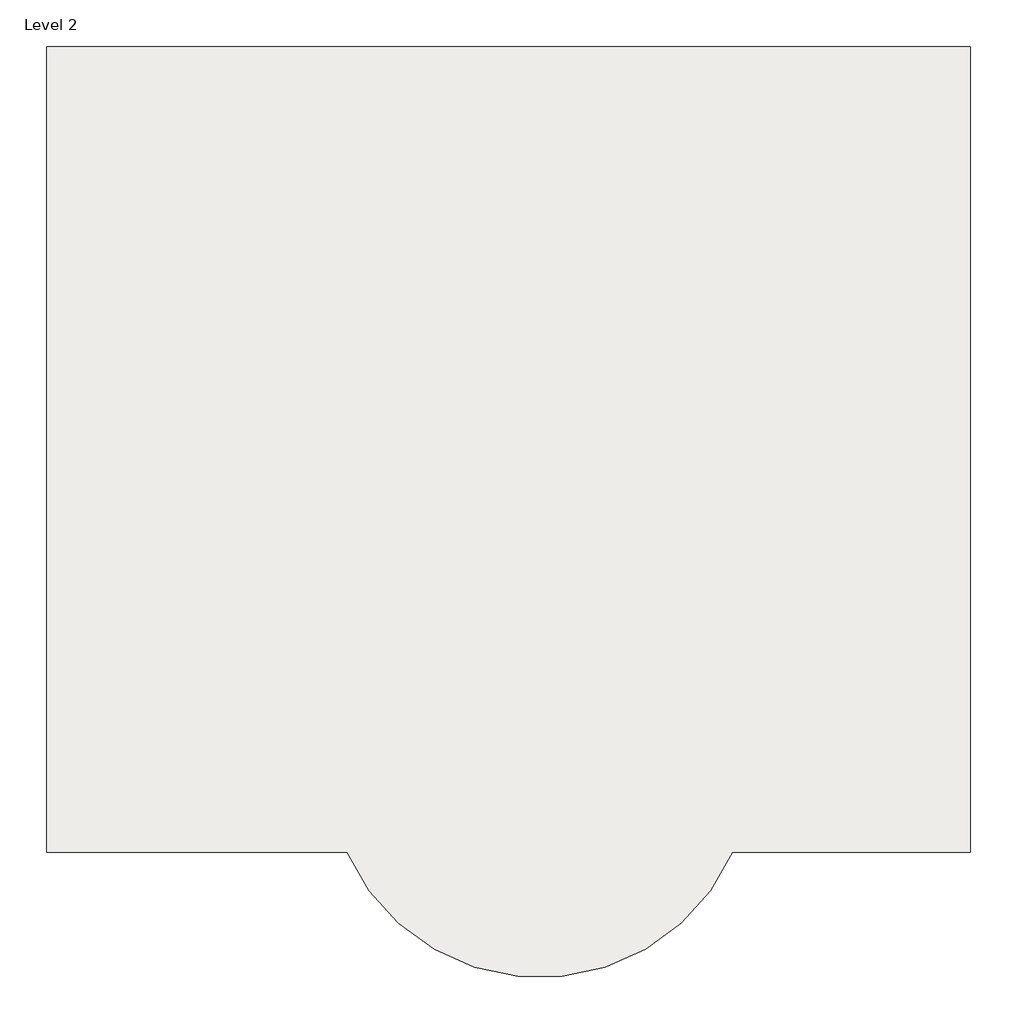
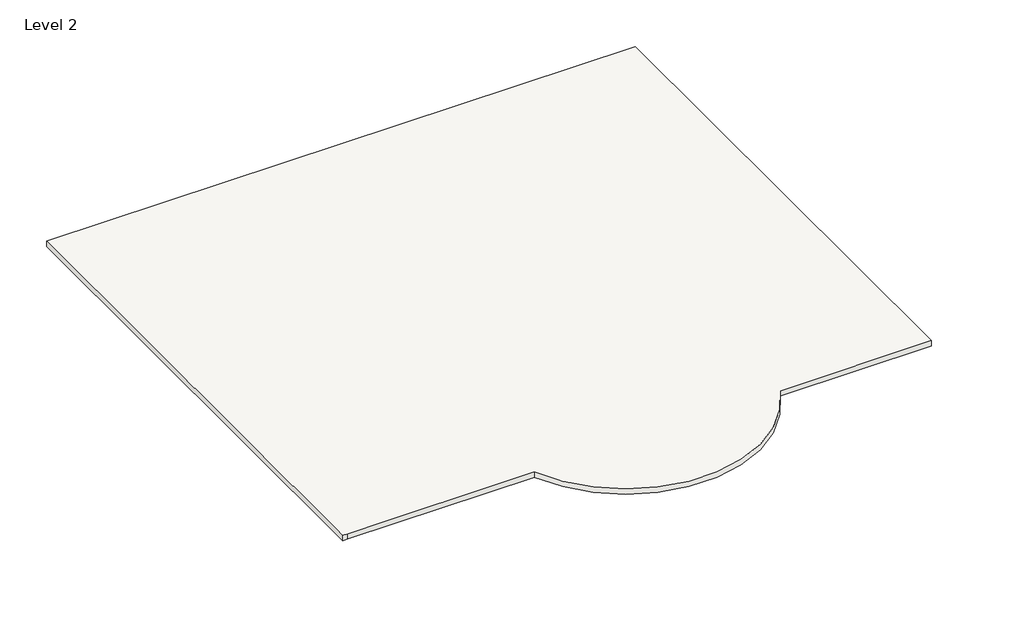
# One storey: 1 slab.
"""IFC4 building model written with IfcOpenShell, lengths in millimetres."""

from ifc_helpers import new_model, si_unit, point, frame, frame_2d, origin, place, context, project, spatial, polyline, circle_curve, trimmed, segment, composite_curve, outline, extrude, element, save

model = new_model("IFC4")

# Units and contexts
model_context = context("Model", 3, world=origin())
ifc_project = project(units=[si_unit("LENGTHUNIT", "METRE", prefix="MILLI")], contexts=[model_context])

# Site, building, storey
site = spatial("IfcSite", under=ifc_project)
building = spatial("IfcBuilding", under=site)
storey = spatial("IfcBuildingStorey", under=building, Name="Level 2", Elevation=3048.0)

# Slab
placement = place(None, origin())
element("IfcSlab", 1, ObjectType="9\"", at=placement, inside=storey, context=model_context, shape_type="SweptSolid", body=[
    extrude(outline(composite_curve([segment(polyline([(-16607.9505427, 7359.5191779), (7979.2494573, 7359.5191779), (7979.2494573, -14078.0808221), (1652.8739931, -14078.0808221)]), True, "CONTINUOUS"), segment(trimmed(circle_curve(frame_2d((-3476.1505427, -11788.3650223)), 5616.9111737), [point((1652.8739931, -14078.0808221))], [point((-8605.1750786, -14078.0808221))], False, "CARTESIAN"), True, "CONTINUOUS"), segment(polyline([(-8605.1750786, -14078.0808221), (-16404.7505427, -14078.0808221), (-16607.9505427, -14078.0808221), (-16607.9505427, 7359.5191779)]), True, "CONTINUOUS")], self_intersect=False)), frame((0.0, 0.0, 3048.0), z_axis=(0.0, 0.0, 1.0), x_axis=(1.0, 0.0, 0.0)), (0.0, 0.0, 1.0), 228.6),
])

save(model, "model.ifc")

# Revit data of these elements
# Type "9\""
#   Assembly Code = "B1010"
#   Function = 0
#   Layers, outside or top first: 0' - 9" no material (function 1)
# Element 1 (IfcSlab, "9\"")
#   built-in parameter 1001955 = 1.5708 (stored number, unit not read)
#   Height Offset From Level = 0' - 9"
#   Phase Created = New Construction
#   Materials on its faces: "Default Floor"
# Materials
#   "Default Floor": colour RGB 128 128 128, transparency 0
